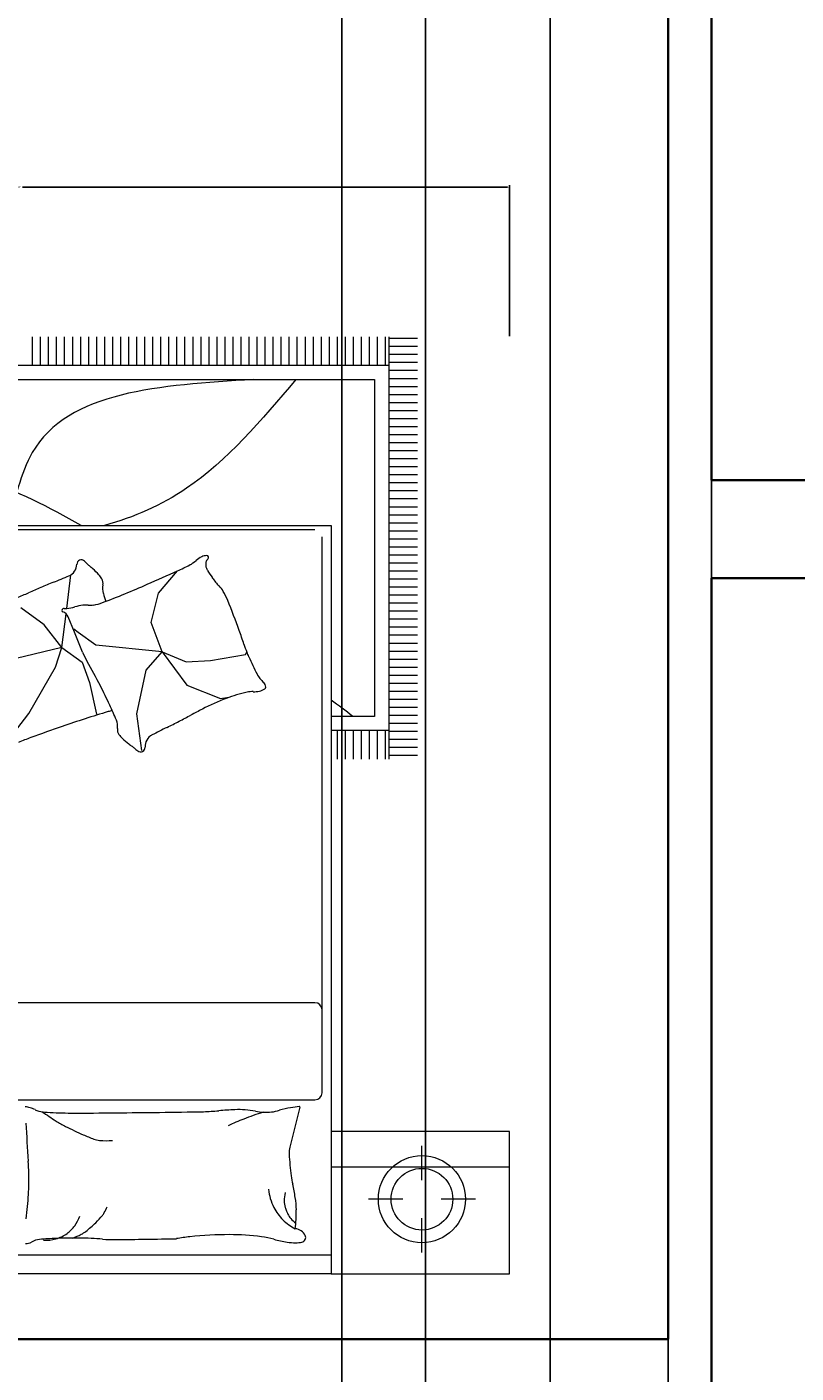
# Model space of a CAD drawing. Units: inches. Extents: x 503 to 1084, y -605 to 132.
# Tile 4 of 14: x 720 to 791, y -437 to -313. Entities that reach past the tile are written whole.
import ezdxf

# ---------------------------------------------------------------- set-up
doc = ezdxf.new("R2010")
doc.units = ezdxf.units.IN
doc.header["$MEASUREMENT"] = 0
doc.layers.add('A-ANNO-DIMS', color=7, linetype='Continuous', lineweight=18)
doc.layers.add('wall', color=1, linetype='Continuous', lineweight=35)
doc.layers.add('furniture', color=50, linetype='Continuous', lineweight=13, transparency=0.8)
doc.styles.add('DIM_FONT', font='SIMPLEX.shx', dxfattribs={"width": 0.8})
doc.styles.get("Standard").update_dxf_attribs({"font": 'arial.ttf'})
doc.dimstyles.get("Standard").update_dxf_attribs({"dimtxt": 0.18, "dimasz": 0.18, "dimexe": 0.18, "dimexo": 0.0625, "dimgap": 0.09, "dimtad": 0, "dimtih": 1, "dimtoh": 1, "dimdec": 1, "dimzin": 0, "dimdsep": 46, "dimlunit": 4, "dimtxsty": 'Standard', "dimcen": 0.09, "dimadec": 0, "dimazin": 0, "dimtfac": 1, "dimtdec": 1, "dimtofl": 0, "dimtmove": 0, "dimatfit": 3, "dimfxl": 1, "dimtolj": 1, "dimtzin": 0, "dimarcsym": 0})

# ---------------------------------------------------------------- blocks, each defined once
blk = doc.blocks.new('A$C4F634EDD')
for p, q in [((0, 2.6295), (0, 2.2295)), ((0.5, 2.6295), (0, 2.6295)), ((0.5, 2.6295), (2.3, 2.6295)), ((0.5, 0.5295), (0.5, 2.6295)), ((0.5, 2.2295), (0.5, 2.6295)), ((0.2457, 2.5697), (0.2457, 2.4733)), ((0.5, 2.5771), (2.3, 2.5771)), ((0.0957, 2.4197), (0.192, 2.4197)), ((0.2994, 2.4197), (0.3957, 2.4197)), ((0.2457, 2.366), (0.2457, 2.2697)), ((0, 2.3301), (0.5, 2.3301)), ((0.5953, 2.1912), (0.616, 2.2738)), ((0, 2.2295), (0.5, 2.2295)), ((0.5878, 2.1612), (0.5953, 2.1912)), ((0.5258, 2.121), (0.5258, 0.5617)), ((1.5035, 2.141), (0.5458, 2.141)), ((0.5458, 1.8684), (1.5653, 1.8684)), ((0.2586, 1.1753), (0.3386, 1.1753)), ((0.3386, 0), (0.3386, 1.1852)), ((0.3486, 1.1052), (0.3486, 1.1852)), ((0.3711, 1.1052), (0.3711, 1.1852)), ((0.3936, 1.1052), (0.3936, 1.1852)), ((0.4161, 1.1052), (0.4161, 1.1852)), ((0.4386, 1.1052), (0.4386, 1.1852)), ((0.4611, 1.1052), (0.4611, 1.1852)), ((0.4836, 1.1052), (0.4836, 1.1852)), ((0.2586, 1.1528), (0.3386, 1.1528)), ((1.031, 1.1612), (1.0448, 1.0581)), ((1.4276, 1.1611), (1.3484, 1.0571)), ((0.2586, 1.1303), (0.3386, 1.1303)), ((0.2586, 1.1078), (0.3386, 1.1078)), ((0.3386, 1.1052), (0.5, 1.1052)), ((0.2586, 1.0853), (0.3386, 1.0853)), ((0.2586, 1.0628), (0.3386, 1.0628)), ((0.3786, 1.0652), (0.5, 1.0652)), ((0.3786, 0.12), (0.3786, 1.0652)), ((1.0448, 1.0581), (1.019, 0.936)), ((1.1784, 0.9702), (1.1586, 1.0591)), ((0.2586, 1.0403), (0.3386, 1.0403)), ((1.3484, 1.0571), (1.2733, 0.9268)), ((0.2586, 1.0178), (0.3386, 1.0178)), ((0.2586, 0.9953), (0.3386, 0.9953)), ((0.8108, 1.0151), (0.7868, 1.0117)), ((0.9054, 0.9773), (0.8108, 1.0151)), ((0.2586, 0.9728), (0.3386, 0.9728)), ((0.2586, 0.9503), (0.3386, 0.9503)), ((0.9743, 0.8845), (0.9054, 0.9773)), ((1.1982, 0.9129), (1.1784, 0.9702)), ((0.2586, 0.9278), (0.3386, 0.9278)), ((0.8384, 0.9085), (0.7403, 0.8913)), ((0.9072, 0.912), (0.8384, 0.9085)), ((0.9743, 0.8845), (0.9072, 0.912)), ((1.019, 0.936), (0.9743, 0.8845)), ((1.2555, 0.8715), (1.1982, 0.9129)), ((1.2733, 0.9268), (1.2555, 0.8715)), ((0.2586, 0.9053), (0.3386, 0.9053)), ((0.2586, 0.8828), (0.3386, 0.8828)), ((0.7403, 0.8913), (0.737, 0.8849)), ((0.9743, 0.8845), (1.0052, 0.802)), ((0.9743, 0.8845), (1.16, 0.8656)), ((1.1973, 0.8853), (1.2203, 0.829)), ((1.2555, 0.8715), (1.2437, 0.7773)), ((1.2555, 0.8715), (1.384, 0.9031)), ((1.2555, 0.8715), (1.3049, 0.8082)), ((0.2586, 0.8603), (0.3386, 0.8603)), ((0.2586, 0.8378), (0.3386, 0.8378)), ((1.16, 0.8656), (1.2099, 0.8295)), ((0.2586, 0.8153), (0.3386, 0.8153)), ((1.0052, 0.802), (0.9846, 0.7194)), ((1.2099, 0.8295), (1.222, 0.8209)), ((1.2203, 0.829), (1.2381, 0.7855)), ((1.3049, 0.8082), (1.3701, 0.7608)), ((0.2586, 0.7928), (0.3386, 0.7928)), ((0.2586, 0.7703), (0.3386, 0.7703)), ((1.2419, 0.7626), (1.23, 0.668)), ((0.2586, 0.7478), (0.3386, 0.7478)), ((0.2586, 0.7253), (0.3386, 0.7253)), ((0.9846, 0.7194), (0.931, 0.6569)), ((0.2586, 0.7028), (0.3386, 0.7028)), ((0.2586, 0.6803), (0.3386, 0.6803)), ((0.2586, 0.6578), (0.3386, 0.6578)), ((0.2586, 0.6353), (0.3386, 0.6353)), ((0.2586, 0.6128), (0.3386, 0.6128)), ((0.2586, 0.5903), (0.3386, 0.5903)), ((0.2586, 0.5678), (0.3386, 0.5678)), ((0.2586, 0.5453), (0.3386, 0.5453)), ((2.3, 0.5295), (0.5, 0.5295)), ((0.5458, 0.5417), (2.2516, 0.5417)), ((0.2586, 0.5228), (0.3386, 0.5228)), ((0.2586, 0.5003), (0.3386, 0.5003)), ((0.2586, 0.4778), (0.3386, 0.4778)), ((0.2586, 0.4553), (0.3386, 0.4553)), ((0.2586, 0.4328), (0.3386, 0.4328)), ((0.2586, 0.4103), (0.3386, 0.4103)), ((0.2586, 0.3878), (0.3386, 0.3878)), ((0.2586, 0.3653), (0.3386, 0.3653)), ((0.2586, 0.3428), (0.3386, 0.3428)), ((0.2586, 0.3203), (0.3386, 0.3203)), ((0.2586, 0.2978), (0.3386, 0.2978)), ((0.2586, 0.2753), (0.3386, 0.2753)), ((0.2586, 0.2528), (0.3386, 0.2528)), ((0.2586, 0.2303), (0.3386, 0.2303)), ((0.2586, 0.2078), (0.3386, 0.2078)), ((0.2586, 0.1853), (0.3386, 0.1853)), ((0.2586, 0.1628), (0.3386, 0.1628)), ((0.2586, 0.1403), (0.3386, 0.1403)), ((0.2586, 0.1178), (0.3386, 0.1178)), ((2.4188, 0.12), (0.3786, 0.12)), ((0.2586, 0.0953), (0.3386, 0.0953)), ((2.4588, 0.08), (0.3386, 0.08)), ((0.3486, 0), (0.3486, 0.08)), ((0.3711, 0), (0.3711, 0.08)), ((0.3936, 0), (0.3936, 0.08)), ((0.4161, 0), (0.4161, 0.08)), ((0.4386, 0), (0.4386, 0.08)), ((0.4611, 0), (0.4611, 0.08)), ((0.4836, 0), (0.4836, 0.08)), ((0.5061, 0), (0.5061, 0.08)), ((0.5286, 0), (0.5286, 0.08)), ((0.5511, 0), (0.5511, 0.08)), ((0.5736, 0), (0.5736, 0.08)), ((0.5961, 0), (0.5961, 0.08)), ((0.6186, 0), (0.6186, 0.08)), ((0.6411, 0), (0.6411, 0.08)), ((0.6636, 0), (0.6636, 0.08)), ((0.6861, 0), (0.6861, 0.08)), ((0.7086, 0), (0.7086, 0.08)), ((0.7311, 0), (0.7311, 0.08)), ((0.7536, 0), (0.7536, 0.08)), ((0.7761, 0), (0.7761, 0.08)), ((0.7986, 0), (0.7986, 0.08)), ((0.8211, 0), (0.8211, 0.08)), ((0.8436, 0), (0.8436, 0.08)), ((0.8661, 0), (0.8661, 0.08)), ((0.8886, 0), (0.8886, 0.08)), ((0.9111, 0), (0.9111, 0.08)), ((0.9336, 0), (0.9336, 0.08)), ((0.9561, 0), (0.9561, 0.08)), ((0.9786, 0), (0.9786, 0.08)), ((1.0011, 0), (1.0011, 0.08)), ((1.0236, 0), (1.0236, 0.08)), ((1.0461, 0), (1.0461, 0.08)), ((1.0686, 0), (1.0686, 0.08)), ((1.0911, 0), (1.0911, 0.08)), ((1.1136, 0), (1.1136, 0.08)), ((1.1361, 0), (1.1361, 0.08)), ((1.1586, 0), (1.1586, 0.08)), ((1.1811, 0), (1.1811, 0.08)), ((1.2036, 0), (1.2036, 0.08)), ((1.2261, 0), (1.2261, 0.08)), ((1.2486, 0), (1.2486, 0.08)), ((1.2711, 0), (1.2711, 0.08)), ((1.2936, 0), (1.2936, 0.08)), ((1.3161, 0), (1.3161, 0.08)), ((1.3386, 0), (1.3386, 0.08)), ((0.2586, 0.0728), (0.3386, 0.0728)), ((0.2586, 0.0503), (0.3386, 0.0503)), ((0.2586, 0.0278), (0.3386, 0.0278)), ((0.2586, 0.0053), (0.3386, 0.0053))]:
    blk.add_line(p, q)
for radius in [0.1222, 0.0865]:
    blk.add_circle((0.2457, 2.4197), radius)
for centre, radius, start, end in [((0.5848, 2.5274), 0.0131, 101.2724, 206.5805), ((0.5999, 2.4516), 0.0904, 90, 101.2724), ((0.5999, 2.3808), 0.1611, 81.5628, 90), ((0.5788, 2.2388), 0.3048, 74.256, 81.5628), ((0.7272, 2.7653), 0.2422, 254.256, 262.4531), ((0.8402, 3.0514), 0.5293, 276.0867, 280.1899), ((1.1602, -8.1346), 10.6675, 90.30153, 91.21582), ((1.1169, 2.2433), 0.2897, 85.1982, 92.5386), ((1.2142, 3.4021), 0.8732, 265.1982, 269.4243), ((1.2995, 2.4357), 0.0992, 105.9352, 126.0864), ((1.2429, 3.3501), 0.8208, 271.9079, 275.2592), ((1.2995, 2.4357), 0.0992, 85.7841, 105.9352), ((1.3132, 2.5864), 0.0539, 275.2592, 300.6513), ((1.3554, 2.5152), 0.0289, 85.6975, 120.6513), ((0.6036, 2.5368), 0.0342, 206.5805, 265.5998), ((1.0898, 2.4496), 0.4918, 173.7676, 180), ((0.5368, 2.3783), 0.1399, 45.0976, 62.7964), ((0.7851, 3.2019), 0.6827, 262.4531, 270), ((0.7851, 3.5682), 1.049, 270, 276.0867), ((1.4317, 2.2032), 0.3916, 128.3886, 133.8115), ((1.2362, 2.45), 0.0768, 117.2396, 128.3886), ((1.3082, 2.3102), 0.234, 110.8603, 117.2396), ((1.2204, 4.0232), 1.4943, 269.4243, 271.9079), ((1.2995, 2.4357), 0.0992, 143.8234, 161.5603), ((1.2995, 2.4357), 0.0992, 126.0864, 143.8234), ((0.5462, 2.4142), 0.0899, 41.4429, 53.7359), ((0.5741, 2.4389), 0.0526, 25.3551, 41.4429), ((0.4851, 2.3967), 0.1511, 21.8149, 25.3551), ((0.5368, 2.3783), 0.1399, 27.3988, 45.0976), ((1.3127, 2.3625), 0.2002, 151.6832, 156.9972), ((1.1799, 2.4341), 0.0493, 140.9651, 151.6832), ((1.3165, 2.3233), 0.2252, 133.8115, 140.9651), ((2.2605, 2.3525), 0.9131, 172.3191, 176.6313), ((0.8019, 2.4496), 0.204, 180, 189.6844), ((0.4345, 2.3765), 0.2056, 18.7799, 21.8149), ((0.576, 2.4246), 0.0562, 0, 18.7799), ((0.5406, 2.4246), 0.0915, 345.3149, 0), ((0.5368, 2.3783), 0.1399, 16.515, 27.3988), ((0.5368, 2.3783), 0.1399, 5.6311, 16.515), ((1.4703, 2.5637), 0.882, 189.6844, 192.1984), ((2.0266, 2.3663), 0.6787, 176.6313, 181.6331), ((0.2982, 2.3103), 0.3171, 8.0051, 12.1984), ((-0.0401, 2.2627), 0.6588, 2.6649, 8.0051), ((2.7128, 2.3859), 1.3652, 181.6331, 183.055), ((14.9657, 3.0398), 13.6356, 183.05496, 183.50486), ((0.5503, 2.2902), 0.0677, 345.9548, 2.6649), ((1.1303, 1.9835), 0.2721, 85.9172, 93.5552), ((1.1455, 2.197), 0.058, 69.3257, 85.9172), ((0.9871, 1.7772), 0.5066, 65.6735, 69.3257), ((0.6058, 0.9338), 1.4323, 63.5015, 65.6735), ((0.473, 2.8815), 0.7387, 289.428, 291.6577), ((0.473, 2.8815), 0.7387, 291.6577, 293.4844), ((0.473, 2.8815), 0.7387, 293.4844, 295.3111), ((1.1054, 1.9358), 0.3126, 57.865, 63.5015), ((0.8841, 1.5835), 0.7286, 54.1737, 57.865), ((0.5887, 2.1609), 0.000917, 165.9551, 274.0829), ((0.5695, 2.4301), 0.2708, 274.0829, 279.4841), ((0.5763, 2.3896), 0.2297, 279.4841, 287.3864), ((0.6807, 2.0561), 0.1197, 96.4341, 107.3864), ((0.6836, 2.0301), 0.1459, 78.4414, 96.4341), ((0.473, 2.8815), 0.7387, 287.1982, 289.428), ((0.759, 2.3985), 0.2301, 258.4414, 272.7491), ((0.7026, 3.5718), 1.4048, 272.7491, 274.6176), ((0.9136, 0.9591), 1.2165, 92.6096, 94.6176), ((1.2501, -19.8405), 22.0183, 90.37908, 91.01965), ((1.2012, -3.5404), 5.7185, 89.7135, 90.9704), ((1.224, 1.0141), 1.164, 86.426, 89.7135), ((1.2875, 2.0302), 0.1459, 77.131, 86.426), ((1.3099, 2.1283), 0.0453, 62.7159, 77.131), ((1.3658, 2.2367), 0.0767, 242.7159, 253.7788), ((1.3688, 2.247), 0.0875, 253.7788, 262.8796), ((0.5458, 2.121), 0.02, 90, 180), ((0.5458, 1.8884), 0.02, 180, 270), ((0.9863, 1.1494), 0.0359, 297.2902, 3.2455), ((1.0348, 1.1521), 0.0127, 51.1864, 183.2455), ((0.9991, 1.1077), 0.0697, 45.8726, 51.1864), ((1.0791, 1.1902), 0.0452, 225.8726, 232.4713), ((1.2846, 1.4577), 0.3825, 232.4713, 233.7837), ((0.6683, 0.6162), 0.6605, 52.7849, 53.7837), ((0.9362, 0.9689), 0.2176, 46.4776, 52.7849), ((1.0543, 1.9106), 0.8371, 290.1287, 292.7069), ((1.8575, -0.7096), 2.0162, 116.4147, 117.4999), ((-0.4173, 3.8699), 3.0972, 296.4147, 297.2902), ((1.0327, 1.0706), 0.0774, 35.8936, 46.4776), ((1.0771, 1.1027), 0.0226, 351.9508, 35.8936), ((1.1449, 1.0931), 0.0458, 171.9508, 202.4162), ((-0.4107, 5.9078), 5.0942, 289.0836, 290.1287), ((-1.8336, 6.2238), 5.8383, 297.49208, 297.84822), ((3.744, -4.3336), 6.1019, 117.49986, 117.84822), ((2.032, 1.4591), 1.0054, 202.4162, 205.0529), ((0.2266, 4.0657), 3.145, 286.6085, 289.0836), ((0.5736, 1.5979), 0.6236, 290.7486, 297.4921), ((1.0922, 1.1636), 0.1166, 280.7366, 286.6085), ((2.6493, 1.7476), 1.6868, 205.0529, 207.0884), ((0.6894, 0.9832), 0.0058, 121.6917, 179.0386), ((0.7004, 0.983), 0.0168, 179.0386, 229.4914), ((0.7131, 0.9448), 0.0509, 103.0402, 121.6917), ((0.7152, 0.9361), 0.0599, 86.6119, 103.0402), ((0.7224, 1.0587), 0.063, 266.6119, 282.6252), ((0.6422, 1.4168), 0.43, 282.6252, 290.7486), ((0.6405, 0.9128), 0.0755, 26.3332, 49.4914), ((-1.6775, -0.2344), 2.6619, 25.1732, 26.3332), ((2.541, 1.6922), 1.5652, 207.0884, 209.936), ((0.9989, 0.8042), 0.2143, 22.2355, 29.936), ((0.5689, 0.8213), 0.1798, 20.7081, 25.1732), ((0.2268, 0.692), 0.5454, 18.2369, 20.7081), ((2.3102, 1.3785), 1.6481, 198.2369, 199.6584), ((2.6444, 1.4979), 2.003, 199.6584, 202.2355), ((1.1727, 0.9313), 0.1794, 277.6784, 284.8807), ((1.2689, 0.569), 0.1955, 97.9822, 104.8807), ((1.2594, 0.7942), 0.0231, 202.2355, 252.8133), ((1.2465, 0.729), 0.034, 85.7407, 97.9822), ((1.2497, 0.772), 0.0092, 265.7407, 289.3799), ((1.2512, 0.7678), 0.00467, 289.3799, 72.8133), ((0.9722, 0.8143), 0.1965, 202.2355, 210.4694), ((2.2689, -2.1899), 3.145, 111.0043, 113.4795), ((0.1831, 0.4093), 1.0054, 18.0203, 19.3448), ((1.0957, 0.7061), 0.0458, 347.5549, 18.0203), ((1.1834, 0.6373), 0.1166, 98.1216, 111.0043), ((1.1763, 0.687), 0.0663, 85.4882, 98.1216), ((1.1871, 0.8241), 0.0712, 265.4882, 277.6784), ((-1.0798, 6.3161), 6.1019, 293.10398, 293.45234), ((3.6722, -4.6377), 5.8383, 113.0962, 113.45234), ((0.8727, 0.7557), 0.081, 210.4694, 224.0964), ((0.6752, 0.5644), 0.194, 35.3015, 44.0964), ((3.0455, -3.9778), 5.0942, 113.4795, 114.5246), ((1.1625, 0.6914), 0.0226, 167.5549, 211.4977), ((2.4404, -2.1823), 3.0972, 112.0188, 112.8944), ((0.5234, 2.5582), 2.0162, 292.0188, 293.104), ((0.5462, 0.4731), 0.352, 31.2138, 35.3015), ((0.8136, 0.6351), 0.0393, 18.9668, 31.2138), ((0.8364, 0.6429), 0.0153, 1.6673, 18.9668), ((0.7746, 0.6411), 0.0771, 353.9885, 1.6673), ((1.2784, -0.1047), 0.8371, 114.5246, 117.1028), ((1.2092, 0.72), 0.0774, 211.4977, 222.0817), ((1.3133, 0.814), 0.2176, 222.0817, 228.389), ((1.6074, 1.1451), 0.6605, 228.389, 229.3878), ((0.9284, 0.3533), 0.3825, 48.0754, 49.3878), ((1.2495, 0.6379), 0.0359, 112.8944, 178.8496), ((0.8506, 0.6191), 0.0063, 130.9751, 197.6767), ((0.8488, 0.6185), 0.00443, 197.6767, 270.4475), ((0.8372, 0.6345), 0.0142, 310.9751, 353.9885), ((0.8486, 0.6493), 0.0352, 270.4475, 294.7411), ((0.8382, 0.6719), 0.0601, 294.7411, 312.9813), ((0.9332, 0.57), 0.0792, 117.1028, 132.9813), ((1.1538, 0.6043), 0.0452, 41.4767, 48.0754), ((1.2399, 0.6804), 0.0697, 221.4767, 226.7905), ((1.2009, 0.6389), 0.0127, 226.7905, 358.8496)]:
    blk.add_arc(centre, radius, start, end)
blk.add_open_spline([(0.4393, 1.0652), (0.4595, 1.05), (0.4798, 1.0348), (0.5, 1.0195)], degree=3)
for points, knots in [([(0.5992, 0.12), (0.6957, 0.2341), (0.8523, 0.4189), (1.0536, 0.5069), (1.136, 0.5295)], [0, 0, 0, 0, 432.822832, 701.445452, 701.445452, 701.445452, 701.445452]), ([(0.7187, 0.12), (0.9791, 0.1362), (1.326, 0.1577), (1.3868, 0.4574), (1.408, 0.5295)], [0, 0, 0, 0, 653.160442, 870.050857, 870.050857, 870.050857, 870.050857]), ([(1.2016, 0.5295), (1.2892, 0.479), (1.5144, 0.3684), (1.8265, 0.2994), (1.9681, 0.4992), (1.9875, 0.5295)], [936.534237, 936.534237, 936.534237, 936.534237, 1243.285375, 1683.261222, 1758.254386, 1758.254386, 1758.254386, 1758.254386])]:
    blk.add_open_spline(points, degree=3, knots=knots)
at = {"style": 'DIM_FONT', "width": 0.8, "flags": 9}
for tag, p in [('YSIZE', (0.5, 2.6295)), ('XSIZE', (0.5, 2.6295)), ('XSIZE', (2.2985, 2.6295)), ('YSIZE', (2.2985, 2.6295))]:
    blk.add_attdef(tag, p, '', height=0.0005, dxfattribs=at)
blk = doc.blocks.new('*D34')
at = {"layer": 'A-ANNO-DIMS', "color": 0, "lineweight": -2, "transparency": 16777216}
for p, q in [((672.72, -341.56), (672.72, -327.68)), ((672.9, -327.86), (717.5, -327.86)), ((764.33, -327.86), (719.73, -327.86)), ((764.51, -341.56), (764.51, -327.68))]:
    blk.add_line(p, q, dxfattribs=at)
at = {"layer": 'A-ANNO-DIMS', "color": 0, "transparency": 16777216}
for points in [[(672.9, -327.83), (672.9, -327.89), (672.72, -327.86)], [(764.33, -327.83), (764.33, -327.89), (764.51, -327.86)]]:
    blk.add_solid(points, dxfattribs=at)
at = {"layer": 'Defpoints', "color": 0, "transparency": 16777216}
for p in [(672.72, -327.86), (672.72, -341.62), (764.51, -341.62)]:
    blk.add_point(p, dxfattribs=at)
at = {"layer": 'A-ANNO-DIMS', "color": 0, "transparency": 16777216, "insert": (718.62, -327.86), "char_height": 0.18, "attachment_point": 5}
blk.add_mtext('\\A1;BED GROUP 7\'-8"', dxfattribs=at)
blk = doc.blocks.new('*D48')
at = {"layer": 'A-ANNO-DIMS', "color": 0, "lineweight": -2, "transparency": 16777216}
for p, q in [((783.09, -354.75), (783.09, 43.51)), ((783.27, 43.33), (789.22, 43.33)), ((795.82, 43.33), (789.86, 43.33)), ((796, -354.75), (796, 43.51))]:
    blk.add_line(p, q, dxfattribs=at)
at = {"layer": 'A-ANNO-DIMS', "color": 0, "transparency": 16777216}
for points in [[(783.27, 43.36), (783.27, 43.3), (783.09, 43.33)], [(795.82, 43.36), (795.82, 43.3), (796, 43.33)]]:
    blk.add_solid(points, dxfattribs=at)
at = {"layer": 'Defpoints', "color": 0, "transparency": 16777216}
for p in [(796, 43.33), (783.09, -354.82), (796, -354.82)]:
    blk.add_point(p, dxfattribs=at)
at = {"layer": 'A-ANNO-DIMS', "color": 0, "transparency": 16777216, "insert": (789.54, 43.33), "char_height": 0.18, "attachment_point": 5}
blk.add_mtext('\\A1;1\'-1"', dxfattribs=at)
blk = doc.blocks.new('*D60')
at = {"layer": 'A-ANNO-DIMS', "color": 0, "lineweight": -2, "transparency": 16777216}
for p, q in [((749.09, -117.88), (749.09, -583.15)), ((779.09, -117.88), (779.09, -583.15)), ((749.27, -582.97), (763.76, -582.97)), ((778.91, -582.97), (764.42, -582.97))]:
    blk.add_line(p, q, dxfattribs=at)
at = {"layer": 'A-ANNO-DIMS', "color": 0, "transparency": 16777216}
for points in [[(749.27, -582.94), (749.27, -583), (749.09, -582.97)], [(778.91, -582.94), (778.91, -583), (779.09, -582.97)]]:
    blk.add_solid(points, dxfattribs=at)
at = {"layer": 'Defpoints', "color": 0, "transparency": 16777216}
for p in [(749.09, -117.82), (779.09, -117.82), (779.09, -582.97)]:
    blk.add_point(p, dxfattribs=at)
at = {"layer": 'A-ANNO-DIMS', "color": 0, "transparency": 16777216, "insert": (764.09, -582.97), "char_height": 0.18, "attachment_point": 5}
blk.add_mtext('\\A1;2\'-6"', dxfattribs=at)
blk = doc.blocks.new('*D63')
at = {"layer": 'A-ANNO-DIMS', "color": 0, "lineweight": -2, "transparency": 16777216}
for p, q in [((783.15, -281.32), (1083.42, -281.32)), ((1083.24, -281.5), (1083.24, -317.88)), ((1083.24, -354.64), (1083.24, -318.25)), ((783.15, -354.82), (1083.42, -354.82))]:
    blk.add_line(p, q, dxfattribs=at)
at = {"layer": 'A-ANNO-DIMS', "color": 0, "transparency": 16777216}
for points in [[(1083.21, -281.5), (1083.27, -281.5), (1083.24, -281.32)], [(1083.21, -354.64), (1083.27, -354.64), (1083.24, -354.82)]]:
    blk.add_solid(points, dxfattribs=at)
at = {"layer": 'Defpoints', "color": 0, "transparency": 16777216}
for p in [(783.09, -281.32), (783.09, -354.82), (1083.24, -354.82)]:
    blk.add_point(p, dxfattribs=at)
at = {"layer": 'A-ANNO-DIMS', "color": 0, "transparency": 16777216, "insert": (1083.24, -318.07), "char_height": 0.18, "attachment_point": 5}
blk.add_mtext('\\A1;6\'-1 1/2"', dxfattribs=at)
blk = doc.blocks.new('*D68')
at = {"layer": 'A-ANNO-DIMS', "color": 0, "lineweight": -2, "transparency": 16777216}
for p, q in [((779.09, -117.88), (779.09, -583.15)), ((783.09, -117.88), (783.09, -583.15)), ((779.27, -582.97), (780.76, -582.97)), ((782.91, -582.97), (781.42, -582.97))]:
    blk.add_line(p, q, dxfattribs=at)
at = {"layer": 'A-ANNO-DIMS', "color": 0, "transparency": 16777216}
for points in [[(779.27, -582.94), (779.27, -583), (779.09, -582.97)], [(782.91, -582.94), (782.91, -583), (783.09, -582.97)]]:
    blk.add_solid(points, dxfattribs=at)
at = {"layer": 'Defpoints', "color": 0, "transparency": 16777216}
for p in [(779.09, -117.82), (783.09, -117.82), (783.09, -582.97)]:
    blk.add_point(p, dxfattribs=at)
at = {"layer": 'A-ANNO-DIMS', "color": 0, "transparency": 16777216, "insert": (781.09, -582.97), "char_height": 0.18, "attachment_point": 5}
blk.add_mtext('\\A1;0\'-4"', dxfattribs=at)
blk = doc.blocks.new('*D76')
at = {"layer": 'A-ANNO-DIMS', "color": 0, "lineweight": -2, "transparency": 16777216}
for p, q in [((756.77, -45.47), (756.77, -583.15)), ((768.24, -45.47), (768.24, -583.15)), ((756.95, -582.97), (761.9, -582.97)), ((768.06, -582.97), (763.11, -582.97))]:
    blk.add_line(p, q, dxfattribs=at)
at = {"layer": 'A-ANNO-DIMS', "color": 0, "transparency": 16777216}
for points in [[(756.95, -582.94), (756.95, -583), (756.77, -582.97)], [(768.06, -582.94), (768.06, -583), (768.24, -582.97)]]:
    blk.add_solid(points, dxfattribs=at)
at = {"layer": 'Defpoints', "color": 0, "transparency": 16777216}
for p in [(756.77, -45.4), (768.24, -45.4), (768.24, -582.97)]:
    blk.add_point(p, dxfattribs=at)
at = {"layer": 'A-ANNO-DIMS', "color": 0, "transparency": 16777216, "insert": (762.51, -582.97), "char_height": 0.18, "attachment_point": 5}
blk.add_mtext('\\A1;0\'-11 1/2"', dxfattribs=at)

msp = doc.modelspace()

# ---------------------------------------------------------------- linework, layer by layer
at = {"layer": 'wall'}
for p, q in [((779.09, -281.32), (779.09, -433.82)), ((783.09, -281.32), (783.09, -354.82)), ((783.09, -354.82), (844.09, -354.82)), ((783.09, -363.82), (844.09, -363.82)), ((783.09, -363.82), (783.09, -442.82)), ((659.09, -433.82), (779.09, -433.82))]:
    msp.add_line(p, q, dxfattribs=at)

# ---------------------------------------------------------------- block references
at = {"layer": 'furniture', "xscale": 32.78135669785699, "yscale": 32.78135669785699, "zscale": 32.78135669785699, "rotation": 180}
msp.add_blockref('A$C4F634EDD', (764.51, -341.62), dxfattribs=at)

# ---------------------------------------------------------------- dimensions: what is measured, and where the dimension line sits
at = {"layer": 'A-ANNO-DIMS'}
for base, p1, p2, picture, middle in [((796, 43.33), (783.09, -354.82), (796, -354.82), '*D48', (789.54, 43.33)), ((768.24, -582.97), (756.77, -45.4), (768.24, -45.4), '*D76', (762.51, -582.97)), ((779.09, -582.97), (749.09, -117.82), (779.09, -117.82), '*D60', (764.09, -582.97)), ((783.09, -582.97), (779.09, -117.82), (783.09, -117.82), '*D68', (781.09, -582.97))]:
    dim = msp.add_linear_dim(base=base, p1=p1, p2=p2, dimstyle='Standard', override={"dimdec": 1, "dimlfac": 1, "dimrnd": 0, "dimzin": 1, "dimdsep": 46, "dimlunit": 4, "dimfrac": 2}, dxfattribs=at)
    dim.commit()
    dim.dimension.update_dxf_attribs({"geometry": picture, "text_midpoint": middle})
dim = msp.add_linear_dim(base=(1083.24, -354.82), p1=(783.09, -281.32), p2=(783.09, -354.82), angle=90, dimstyle='Standard', override={"dimdec": 1, "dimlfac": 1, "dimrnd": 0, "dimzin": 1, "dimdsep": 46, "dimlunit": 4, "dimfrac": 2}, dxfattribs=at)
dim.commit()
dim.dimension.update_dxf_attribs({"geometry": '*D63', "text_midpoint": (1083.24, -318.07)})
dim = msp.add_linear_dim(base=(672.72, -327.86), p1=(764.51, -341.62), p2=(672.72, -341.62), angle=180, text='BED GROUP <>', dimstyle='Standard', override={"dimdec": 1, "dimlfac": 1, "dimrnd": 0, "dimzin": 1, "dimdsep": 46, "dimlunit": 4, "dimfrac": 2}, dxfattribs=at)
dim.commit()
dim.dimension.update_dxf_attribs({"geometry": '*D34', "text_midpoint": (718.62, -327.86)})

doc.saveas('drawing.dxf')
